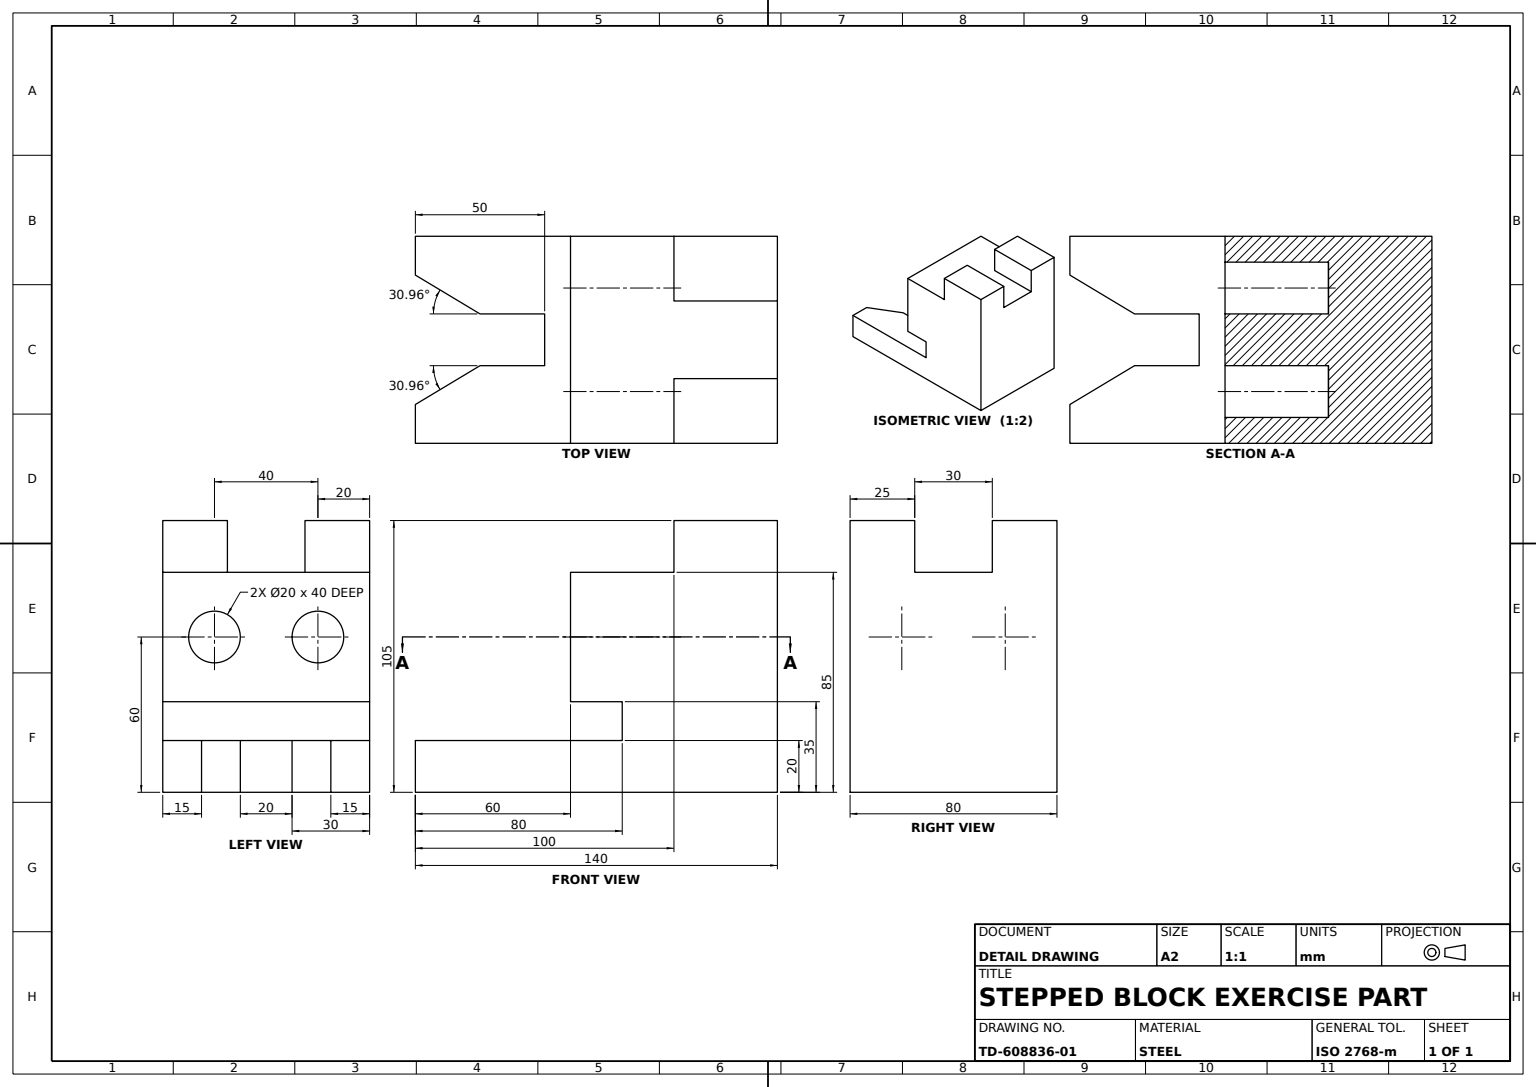
SolidWorks part; units mm, degrees
material "Plain Carbon Steel"
ref_plane "Front Plane" through (0, 0, 0) normal (0, 0, 1) x (1, 0, 0)
ref_plane "Top Plane" through (0, 0, 0) normal (0, 1, 0) x (1, 0, 0)
ref_plane "Right Plane" through (0, 0, 0) normal (1, 0, 0) x (0, 0, -1)
sketch "Base Step Profile Sketch" plane through (0, 0, 0) normal (0, 0, 1) x (1, 0, 0)
  line L0 (0, 0) -> (140, 0)
  line L1 (140, 0) -> (140, 80)
  line L2 (0, 0) -> (0, 20)
  line L3 (0, 20) -> (80, 20)
  line L4 (80, 20) -> (80, 35)
  line L5 (80, 35) -> (60, 35)
  line L6 (60, 35) -> (60, 85)
  line L7 (60, 85) -> (140, 85)
  line L8 (140, 85) -> (140, 80)
  dimension "D1" = 60
  dimension "D2" = 80
  dimension "D3" = 35
  dimension "D4" = 85
extrude "Base Step Body" add sketch "Base Step Profile Sketch" along normal blind 80
sketch "Upper Block Sketch" plane through (0, 0, 80) normal (0, 0, 1) x (1, 0, 0)
  line L0 (140, 85) -> (140, 105)
  line L1 (140, 105) -> (100, 105)
  line L2 (100, 105) -> (100, 85)
  line L3 (100, 85) -> (140, 85)
  line L4 (0, 20) -> (0, 0) construction
  line L5 (0, 0) -> (140, 0) construction
  dimension "D1" = 100
  dimension "D2" = 105
extrude "Upper Block" add sketch "Upper Block Sketch" against normal blind 80
sketch "Corner Notch Sketch 25x25" plane through (0, 105, 0) normal (0, 1, 0) x (1, 0, 0)
  line L0 (100, 0) -> (100, -80) construction
  line L1 (100, -25) -> (140, -25)
  line L2 (100, -25) -> (100, -55)
  line L3 (100, -55) -> (140, -55)
  line L4 (140, -25) -> (140, -55)
  line L5 (140, 0) -> (140, -80) construction
  line L6 (140, 0) -> (100, 0) construction
  line L7 (140, -80) -> (100, -80) construction
  dimension "D1" = 25
  dimension "D2" = 25
extrude "Corner Notch 25x25" cut sketch "Corner Notch Sketch 25x25" against normal blind 20
sketch "Side Recess Sketch" plane through (0, 20, 0) normal (0, 1, 0) x (1, 0, 0)
  line L0 (0, 0) -> (0, -15)
  line L1 (50, -40) -> (50, -50)
  line L2 (0, -80) -> (0, 0) construction
  line L5 (50, -50) -> (25, -50)
  line L6 (50, -40) -> (50, -30)
  line L7 (0, -15) -> (25, -30)
  line L8 (0, -80) -> (0, -65)
  line L9 (0, -65) -> (25, -50)
  line L10 (50, -30) -> (25, -30)
  line L11 (80, 0) -> (0, 0) construction
  dimension "D1" = 25
  dimension "D2" = 50
  dimension "D3" = 15
  dimension "D4" = 30
extrude "Side Recess" cut sketch "Side Recess Sketch" against normal blind 20 and the other way through all
sketch "Slot Sketch" plane through (60, 0, 0) normal (-1, 0, 0) x (0, 0, 1)
  line L0 (80, 85) -> (0, 85) construction
  line L1 (0, 85) -> (0, 35) construction
  circle A0 centre (20, 60) radius 10
  circle A1 centre (60, 60) radius 10
  dimension "D1" = 20
  dimension "D2" = 20
  dimension "D6" = 20
  dimension "D3" = 25
  dimension "D4" = 20
  dimension "D5" = 40
extrude "Slot Cut" cut sketch "Slot Sketch" against normal blind 40
